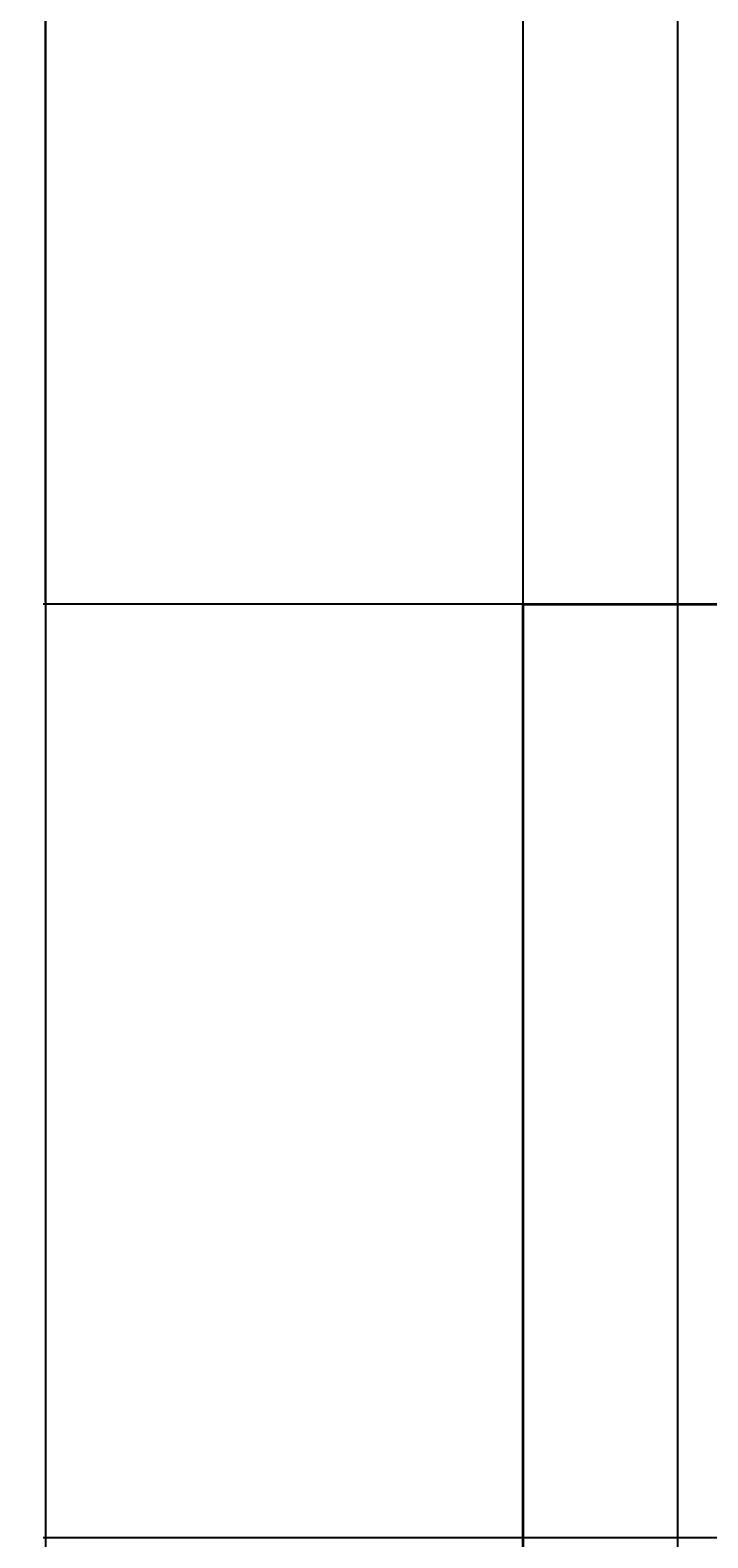
# Model space of a CAD drawing. Units: inches. Extents: x -26 to 776, y -22 to 650.
# Tile 26 of 62: x -26 to 25, y 420 to 535. Entities that reach past the tile are written whole.
import ezdxf

# ---------------------------------------------------------------- set-up
doc = ezdxf.new("R2010")
doc.units = ezdxf.units.IN
doc.header["$MEASUREMENT"] = 0
doc.layers.add('A-ANNO-DIMS', color=2, linetype='Continuous', lineweight=18)
doc.layers.add('A-WALL', color=7, linetype='Continuous', lineweight=35)
doc.styles.get("Standard").update_dxf_attribs({"font": 'arial.ttf'})
doc.dimstyles.get("Standard").update_dxf_attribs({"dimtxt": 0.5625, "dimasz": 0.18, "dimexe": 0.18, "dimexo": 0.0625, "dimgap": 0.09, "dimtad": 0, "dimtih": 1, "dimtoh": 1, "dimdec": 4, "dimzin": 0, "dimdsep": 46, "dimlunit": 4, "dimtxsty": 'Standard', "dimcen": 0.09, "dimadec": 0, "dimazin": 0, "dimtfac": 1, "dimtdec": 4, "dimtofl": 0, "dimtmove": 0, "dimatfit": 3, "dimfxl": 1, "dimtolj": 1, "dimtzin": 0, "dimarcsym": 0})

# ---------------------------------------------------------------- blocks, each defined once
blk = doc.blocks.new('*D14')
at = {"layer": 'A-ANNO-DIMS', "color": 0, "lineweight": -2, "transparency": 16777216}
for p, q in [((191.62, 613.27), (-25.48, 613.27)), ((-25.3, 613.09), (-25.3, 314.75)), ((-25.3, 15.66), (-25.3, 314)), ((11.04, 15.48), (-25.48, 15.48))]:
    blk.add_line(p, q, dxfattribs=at)
at = {"layer": 'A-ANNO-DIMS', "color": 0, "transparency": 16777216}
for points in [[(-25.33, 613.09), (-25.27, 613.09), (-25.3, 613.27)], [(-25.33, 15.66), (-25.27, 15.66), (-25.3, 15.48)]]:
    blk.add_solid(points, dxfattribs=at)
at = {"layer": 'Defpoints', "color": 0, "transparency": 16777216}
for p in [(-25.3, 613.27), (191.68, 613.27), (11.11, 15.48)]:
    blk.add_point(p, dxfattribs=at)
at = {"layer": 'A-ANNO-DIMS', "color": 0, "transparency": 16777216, "insert": (-25.3, 314.38), "char_height": 0.562, "attachment_point": 5}
blk.add_mtext('\\A1;597.8', dxfattribs=at)
blk = doc.blocks.new('*D15')
at = {"layer": 'A-ANNO-DIMS', "color": 0, "lineweight": -2, "transparency": 16777216}
for p, q in [((11.11, 491.49), (11.11, 649.86)), ((11.29, 649.68), (120.22, 649.68)), ((231.24, 649.68), (122.31, 649.68)), ((231.42, 491.49), (231.42, 649.86))]:
    blk.add_line(p, q, dxfattribs=at)
at = {"layer": 'A-ANNO-DIMS', "color": 0, "transparency": 16777216}
for points in [[(11.29, 649.71), (11.29, 649.65), (11.11, 649.68)], [(231.24, 649.71), (231.24, 649.65), (231.42, 649.68)]]:
    blk.add_solid(points, dxfattribs=at)
at = {"layer": 'Defpoints', "color": 0, "transparency": 16777216}
for p in [(231.42, 649.68), (11.11, 491.43), (231.42, 491.43)]:
    blk.add_point(p, dxfattribs=at)
at = {"layer": 'A-ANNO-DIMS', "color": 0, "transparency": 16777216, "insert": (121.27, 649.68), "char_height": 0.562, "attachment_point": 5}
blk.add_mtext('\\A1;220.3', dxfattribs=at)
blk = doc.blocks.new('*D17')
at = {"layer": 'A-ANNO-DIMS', "color": 0, "lineweight": -2, "transparency": 16777216}
for p, q in [((11.11, 491.49), (11.11, 649.86)), ((11.29, 649.68), (100.16, 649.68)), ((191.5, 649.68), (102.62, 649.68)), ((191.68, 613.33), (191.68, 649.86))]:
    blk.add_line(p, q, dxfattribs=at)
at = {"layer": 'A-ANNO-DIMS', "color": 0, "transparency": 16777216}
for points in [[(11.29, 649.71), (11.29, 649.65), (11.11, 649.68)], [(191.5, 649.71), (191.5, 649.65), (191.68, 649.68)]]:
    blk.add_solid(points, dxfattribs=at)
at = {"layer": 'Defpoints', "color": 0, "transparency": 16777216}
for p in [(191.68, 649.68), (191.68, 613.27), (11.11, 491.43)]:
    blk.add_point(p, dxfattribs=at)
at = {"layer": 'A-ANNO-DIMS', "color": 0, "transparency": 16777216, "insert": (101.39, 649.68), "char_height": 0.562, "attachment_point": 5}
blk.add_mtext('\\A1;180.57', dxfattribs=at)
blk = doc.blocks.new('*D19')
at = {"layer": 'A-ANNO-DIMS', "color": 0, "lineweight": -2, "transparency": 16777216}
for p, q in [((191.62, 613.27), (-25.48, 613.27)), ((-25.3, 613.09), (-25.3, 552.73)), ((-25.3, 491.61), (-25.3, 551.97)), ((191.62, 491.43), (-25.48, 491.43))]:
    blk.add_line(p, q, dxfattribs=at)
at = {"layer": 'A-ANNO-DIMS', "color": 0, "transparency": 16777216}
for points in [[(-25.33, 613.09), (-25.27, 613.09), (-25.3, 613.27)], [(-25.33, 491.61), (-25.27, 491.61), (-25.3, 491.43)]]:
    blk.add_solid(points, dxfattribs=at)
at = {"layer": 'Defpoints', "color": 0, "transparency": 16777216}
for p in [(-25.3, 613.27), (191.68, 613.27), (191.68, 491.43)]:
    blk.add_point(p, dxfattribs=at)
at = {"layer": 'A-ANNO-DIMS', "color": 0, "transparency": 16777216, "insert": (-25.3, 552.35), "char_height": 0.562, "attachment_point": 5}
blk.add_mtext('\\A1;121.84', dxfattribs=at)
blk = doc.blocks.new('*D22')
at = {"layer": 'A-ANNO-DIMS', "color": 0, "lineweight": -2, "transparency": 16777216}
for p, q in [((22.89, 15.33), (22.89, 649.86)), ((23.07, 649.68), (119.19, 649.68)), ((217.77, 649.68), (121.65, 649.68)), ((217.95, 15.54), (217.95, 649.86))]:
    blk.add_line(p, q, dxfattribs=at)
at = {"layer": 'A-ANNO-DIMS', "color": 0, "transparency": 16777216}
for points in [[(23.07, 649.71), (23.07, 649.65), (22.89, 649.68)], [(217.77, 649.71), (217.77, 649.65), (217.95, 649.68)]]:
    blk.add_solid(points, dxfattribs=at)
at = {"layer": 'Defpoints', "color": 0, "transparency": 16777216}
for p in [(217.95, 649.68), (22.89, 15.27), (217.95, 15.48)]:
    blk.add_point(p, dxfattribs=at)
at = {"layer": 'A-ANNO-DIMS', "color": 0, "transparency": 16777216, "insert": (120.42, 649.68), "char_height": 0.562, "attachment_point": 5}
blk.add_mtext('\\A1;195.06', dxfattribs=at)
blk = doc.blocks.new('*D24')
at = {"layer": 'A-ANNO-DIMS', "color": 0, "lineweight": -2, "transparency": 16777216}
for p, q in [((11.11, 15.54), (11.11, 649.86)), ((11.29, 649.68), (15.77, 649.68)), ((22.71, 649.68), (18.23, 649.68)), ((22.89, 15.33), (22.89, 649.86))]:
    blk.add_line(p, q, dxfattribs=at)
at = {"layer": 'A-ANNO-DIMS', "color": 0, "transparency": 16777216}
for points in [[(11.29, 649.71), (11.29, 649.65), (11.11, 649.68)], [(22.71, 649.71), (22.71, 649.65), (22.89, 649.68)]]:
    blk.add_solid(points, dxfattribs=at)
at = {"layer": 'Defpoints', "color": 0, "transparency": 16777216}
for p in [(22.89, 649.68), (11.11, 15.48), (22.89, 15.27)]:
    blk.add_point(p, dxfattribs=at)
at = {"layer": 'A-ANNO-DIMS', "color": 0, "transparency": 16777216, "insert": (17, 649.68), "char_height": 0.562, "attachment_point": 5}
blk.add_mtext('\\A1;11.782', dxfattribs=at)
blk = doc.blocks.new('*D25')
at = {"layer": 'A-ANNO-DIMS', "color": 0, "lineweight": -2, "transparency": 16777216}
for p, q in [((11.11, 221.7), (11.11, 649.86)), ((11.29, 649.68), (50.34, 649.68)), ((91.46, 649.68), (52.41, 649.68)), ((91.64, 271.37), (91.64, 649.86))]:
    blk.add_line(p, q, dxfattribs=at)
at = {"layer": 'A-ANNO-DIMS', "color": 0, "transparency": 16777216}
for points in [[(11.29, 649.71), (11.29, 649.65), (11.11, 649.68)], [(91.46, 649.71), (91.46, 649.65), (91.64, 649.68)]]:
    blk.add_solid(points, dxfattribs=at)
at = {"layer": 'Defpoints', "color": 0, "transparency": 16777216}
for p in [(91.64, 649.68), (91.64, 271.31), (11.11, 221.64)]:
    blk.add_point(p, dxfattribs=at)
at = {"layer": 'A-ANNO-DIMS', "color": 0, "transparency": 16777216, "insert": (51.38, 649.68), "char_height": 0.562, "attachment_point": 5}
blk.add_mtext('\\A1;80.54', dxfattribs=at)
blk = doc.blocks.new('*D36')
at = {"layer": 'A-ANNO-DIMS', "color": 0, "lineweight": -2, "transparency": 16777216}
for p, q in [((82.07, 420.28), (-25.48, 420.28)), ((-25.3, 420.1), (-25.3, 290.26)), ((-25.3, 159.66), (-25.3, 289.5)), ((82.07, 159.48), (-25.48, 159.48))]:
    blk.add_line(p, q, dxfattribs=at)
at = {"layer": 'A-ANNO-DIMS', "color": 0, "transparency": 16777216}
for points in [[(-25.33, 420.1), (-25.27, 420.1), (-25.3, 420.28)], [(-25.33, 159.66), (-25.27, 159.66), (-25.3, 159.48)]]:
    blk.add_solid(points, dxfattribs=at)
at = {"layer": 'Defpoints', "color": 0, "transparency": 16777216}
for p in [(-25.3, 420.28), (82.13, 420.28), (82.13, 159.48)]:
    blk.add_point(p, dxfattribs=at)
at = {"layer": 'A-ANNO-DIMS', "color": 0, "transparency": 16777216, "insert": (-25.3, 289.88), "char_height": 0.562, "attachment_point": 5}
blk.add_mtext('\\A1;260.8', dxfattribs=at)

msp = doc.modelspace()

# ---------------------------------------------------------------- linework, layer by layer
at = {"layer": 'A-WALL'}
for p, q in [((11.1074, 491.4269), (231.4249, 491.4269)), ((11.1074, 458.1203), (11.1074, 491.4269)), ((11.1074, 338.1203), (11.1074, 458.1203))]:
    msp.add_line(p, q, dxfattribs=at)

# ---------------------------------------------------------------- dimensions: what is measured, and where the dimension line sits
at = {"layer": 'A-ANNO-DIMS'}
for base, p1, p2, override, picture, middle in [((231.4249, 649.6763), (11.1074, 491.4269), (231.4249, 491.4269), {"dimdec": 1, "dimlfac": 1, "dimrnd": 0, "dimzin": 0, "dimdsep": 46, "dimlunit": 2}, '*D15', (121.2661, 649.6763)), ((191.6782, 649.6763), (11.1074, 491.4269), (191.6782, 613.2713), {"dimdec": 2, "dimlfac": 1, "dimrnd": 0, "dimzin": 0, "dimdsep": 46, "dimlunit": 2}, '*D17', (101.3928, 649.6763)), ((22.8891, 649.6763), (11.1074, 15.4824), (22.8891, 15.2701), {"dimdec": 3, "dimlfac": 1, "dimrnd": 0, "dimzin": 0, "dimdsep": 46, "dimlunit": 2}, '*D24', (16.9982, 649.6763)), ((91.6448, 649.6763), (11.1074, 221.6413), (91.6448, 271.3091), {"dimdec": 2, "dimlfac": 1, "dimrnd": 0, "dimzin": 0, "dimdsep": 46, "dimlunit": 2}, '*D25', (51.3761, 649.6763)), ((217.9529, 649.6763), (22.8891, 15.2701), (217.9529, 15.4824), {"dimdec": 2, "dimlfac": 1, "dimrnd": 0, "dimzin": 0, "dimdsep": 46, "dimlunit": 2}, '*D22', (120.421, 649.6763))]:
    dim = msp.add_linear_dim(base=base, p1=p1, p2=p2, dimstyle='Standard', override=override, dxfattribs=at)
    dim.commit()
    dim.dimension.update_dxf_attribs({"geometry": picture, "text_midpoint": middle})
for base, p1, p2, override, picture, middle in [((-25.2976, 613.2713), (191.6782, 491.4269), (191.6782, 613.2713), {"dimdec": 2, "dimlfac": 1, "dimrnd": 0, "dimzin": 0, "dimdsep": 46, "dimlunit": 2}, '*D19', (-25.2976, 552.3491)), ((-25.2976, 613.2713), (11.1074, 15.4824), (191.6782, 613.2713), {"dimdec": 1, "dimlfac": 1, "dimrnd": 0, "dimzin": 0, "dimdsep": 46, "dimlunit": 2}, '*D14', (-25.2976, 314.3769)), ((-25.2976, 420.2783), (82.134, 159.4824), (82.134, 420.2783), {"dimdec": 1, "dimlfac": 1, "dimrnd": 0, "dimzin": 0, "dimdsep": 46, "dimlunit": 2}, '*D36', (-25.2976, 289.8803))]:
    dim = msp.add_linear_dim(base=base, p1=p1, p2=p2, angle=90, dimstyle='Standard', override=override, dxfattribs=at)
    dim.commit()
    dim.dimension.update_dxf_attribs({"geometry": picture, "text_midpoint": middle})

doc.saveas('drawing.dxf')
